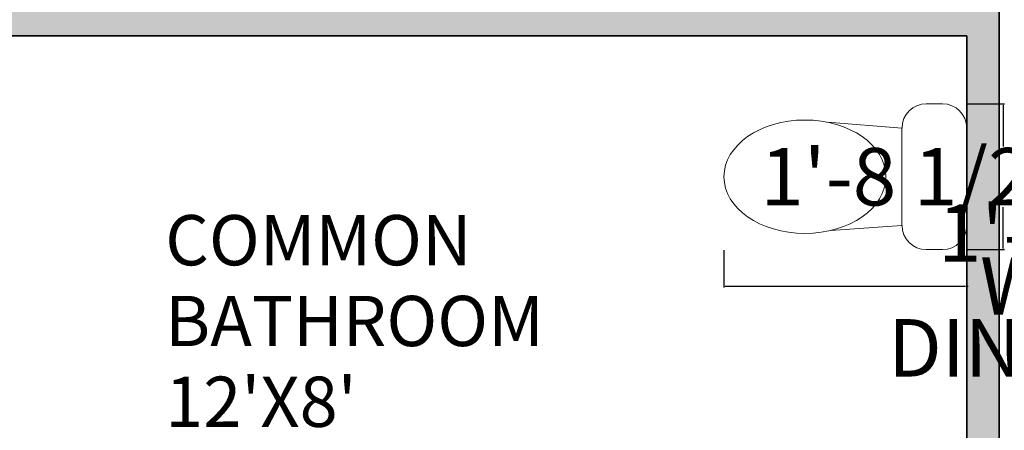
# Model space of a CAD drawing. Units: inches. Extents: x 638 to 1303, y 1 to 699.
# Tile 4 of 21: x 718 to 855, y 252 to 310. Entities that reach past the tile are written whole.
import ezdxf

# ---------------------------------------------------------------- set-up
doc = ezdxf.new("R2010")
doc.units = ezdxf.units.IN
doc.header["$MEASUREMENT"] = 0
for name, color, linetype, lineweight in [('A-ANNO-DIMS', 2, 'Continuous', 18), ('A-AREA-IDEN', 7, 'Continuous', 18), ('A-FLOR-FIXT', 9, 'Continuous', 18), ('A-WALL', 7, 'Continuous', 35)]:
    doc.layers.add(name, color=color, linetype=linetype, lineweight=lineweight)
doc.layers.add('A-WALL-PATT', color=143, linetype='Continuous', lineweight=13, true_color=0x7aafdf)
doc.styles.get("Standard").update_dxf_attribs({"font": 'arial.ttf'})
doc.dimstyles.get("Standard").update_dxf_attribs({"dimtxt": 8, "dimasz": 0.18, "dimexe": 0.18, "dimexo": 0.0625, "dimgap": 0.09, "dimtad": 0, "dimtih": 1, "dimtoh": 1, "dimdec": 4, "dimzin": 0, "dimdsep": 46, "dimlunit": 3, "dimtxsty": 'Standard', "dimcen": 0.09, "dimadec": 0, "dimazin": 0, "dimtfac": 1, "dimtdec": 4, "dimtofl": 0, "dimtmove": 0, "dimatfit": 3, "dimfxl": 1, "dimtolj": 1, "dimtzin": 0, "dimarcsym": 0})

# ---------------------------------------------------------------- blocks, each defined once
blk = doc.blocks.new('WC-CLOSE-COUPLED')
for p, q in [((28.2, 20.3), (30.45, 20.3)), ((24.81, 16.92), (14.41, 17.74)), ((24.81, 3.38), (24.81, 16.92)), ((33.84, 16.92), (33.84, 3.38)), ((24.81, 3.38), (14.9, 2.67)), ((30.45, 0), (28.2, 0))]:
    blk.add_line(p, q)
for centre, start, end in [((28.2, 16.92), 90, 180), ((30.45, 16.92), 0, 90), ((28.2, 3.38), 180, 270), ((30.45, 3.38), 270, 0)]:
    blk.add_arc(centre, 3.38, start, end)
blk.add_ellipse((11.28, 10.15), major_axis=(-11.28, 0), ratio=0.7)
blk = doc.blocks.new('*D30')
at = {"layer": 'A-ANNO-DIMS', "color": 0, "lineweight": -2, "transparency": 16777216}
for p, q in [((913.6, 276.19), (909.79, 276.19)), ((909.97, 276.01), (909.97, 268.11)), ((909.97, 251.76), (909.97, 259.66)), ((913.6, 251.58), (909.79, 251.58))]:
    blk.add_line(p, q, dxfattribs=at)
at = {"layer": 'A-ANNO-DIMS', "color": 0, "transparency": 16777216}
for points in [[(909.94, 276.01), (910, 276.01), (909.97, 276.19)], [(909.94, 251.76), (910, 251.76), (909.97, 251.58)]]:
    blk.add_solid(points, dxfattribs=at)
at = {"layer": 'Defpoints', "color": 0, "transparency": 16777216}
for p in [(913.67, 276.19), (909.97, 251.58), (913.67, 251.58)]:
    blk.add_point(p, dxfattribs=at)
at = {"layer": 'A-ANNO-DIMS', "color": 0, "transparency": 16777216, "insert": (909.97, 263.89), "char_height": 8, "attachment_point": 5}
blk.add_mtext('\\A1;DINING CHAIR 2\'-0 1/2" TYP.', dxfattribs=at)
blk = doc.blocks.new('*D31')
at = {"layer": 'A-ANNO-DIMS', "color": 0, "lineweight": -2, "transparency": 16777216}
for p, q in [((913.67, 279.88), (913.49, 279.88)), ((913.67, 276.25), (913.67, 280.06)), ((934.89, 279.88), (913.85, 279.88)), ((935.07, 276.25), (935.07, 280.06))]:
    blk.add_line(p, q, dxfattribs=at)
at = {"layer": 'A-ANNO-DIMS', "color": 0, "transparency": 16777216}
for points in [[(913.85, 279.91), (913.85, 279.85), (913.67, 279.88)], [(934.89, 279.91), (934.89, 279.85), (935.07, 279.88)]]:
    blk.add_solid(points, dxfattribs=at)
at = {"layer": 'Defpoints', "color": 0, "transparency": 16777216}
for p in [(913.67, 279.88), (913.67, 276.19), (935.07, 276.19)]:
    blk.add_point(p, dxfattribs=at)
at = {"layer": 'A-ANNO-DIMS', "color": 0, "transparency": 16777216, "insert": (880.07, 279.88), "char_height": 8, "attachment_point": 5}
blk.add_mtext('\\A1;1\'-9 1/2" TYP.', dxfattribs=at)
blk = doc.blocks.new('*D32')
at = {"layer": 'A-ANNO-DIMS', "color": 0, "lineweight": -2, "transparency": 16777216}
for p, q in [((816.4, 277.5), (816.4, 272.31)), ((850.23, 277.5), (850.23, 272.31)), ((816.58, 272.49), (850.05, 272.49)), ((850.23, 272.49), (850.41, 272.49))]:
    blk.add_line(p, q, dxfattribs=at)
at = {"layer": 'A-ANNO-DIMS', "color": 0, "transparency": 16777216}
for points in [[(816.58, 272.52), (816.58, 272.46), (816.4, 272.49)], [(850.05, 272.52), (850.05, 272.46), (850.23, 272.49)]]:
    blk.add_solid(points, dxfattribs=at)
at = {"layer": 'Defpoints', "color": 0, "transparency": 16777216}
for p in [(816.4, 277.56), (850.23, 277.56), (850.23, 272.49)]:
    blk.add_point(p, dxfattribs=at)
at = {"layer": 'A-ANNO-DIMS', "color": 0, "transparency": 16777216, "insert": (889.02, 272.49), "char_height": 8, "attachment_point": 5}
blk.add_mtext('\\A1;WC 2\'-10" TYP.', dxfattribs=at)
blk = doc.blocks.new('*D33')
at = {"layer": 'A-ANNO-DIMS', "color": 0, "lineweight": -2, "transparency": 16777216}
for p, q in [((850.3, 297.86), (855.49, 297.86)), ((855.31, 297.68), (855.31, 291.94)), ((855.31, 277.74), (855.31, 283.49)), ((850.3, 277.56), (855.49, 277.56))]:
    blk.add_line(p, q, dxfattribs=at)
at = {"layer": 'A-ANNO-DIMS', "color": 0, "transparency": 16777216}
for points in [[(855.28, 297.68), (855.34, 297.68), (855.31, 297.86)], [(855.28, 277.74), (855.34, 277.74), (855.31, 277.56)]]:
    blk.add_solid(points, dxfattribs=at)
at = {"layer": 'Defpoints', "color": 0, "transparency": 16777216}
for p in [(850.23, 297.86), (855.31, 297.86), (850.23, 277.56)]:
    blk.add_point(p, dxfattribs=at)
at = {"layer": 'A-ANNO-DIMS', "color": 0, "transparency": 16777216, "insert": (855.31, 287.71), "char_height": 8, "attachment_point": 5}
blk.add_mtext('\\A1;1\'-8 1/2" TYP.', dxfattribs=at)

msp = doc.modelspace()

# ---------------------------------------------------------------- hatches: boundary and pattern name
at = {"layer": 'A-WALL-PATT'}
h = msp.add_hatch(color=256, dxfattribs=at)
h.dxf.hatch_style = 1
h.paths.add_polyline_path([(973.34524, 629.81895), (793.35541, 629.81895), (793.35541, 620.81895), (850.23798, 620.81895), (922.23798, 620.81895), (922.23798, 524.81895), (908.94335, 524.81895), (908.94335, 520.31895), (926.73798, 520.31895), (926.73798, 544.31895), (979.3571, 544.31895), (979.3571, 548.81895), (926.73798, 548.81895), (926.73798, 620.81895), (973.34524, 620.81895)])
h.paths.add_polyline_path([(758.35541, 629.81895), (697.23798, 629.81895), (697.23798, 586.77451), (706.23798, 586.77451), (706.23798, 620.81895), (758.35541, 620.81895)])
h.paths.add_polyline_path([(1075.85281, 629.81895), (1003.34524, 629.81895), (1003.34524, 620.81895), (1046.73798, 620.81895), (1046.73798, 560.81895), (1046.73798, 548.81895), (1026.3571, 548.81895), (1026.3571, 544.31895), (1046.73798, 544.31895), (1046.73798, 486.87457), (1051.23798, 486.87457), (1051.23798, 556.31895), (1162.89753, 556.31895), (1162.89753, 560.81895), (1051.23798, 560.81895), (1051.23798, 620.81895), (1075.85281, 620.81895)])
h.paths.add_polyline_path([(1228.23798, 629.81895), (1105.85281, 629.81895), (1105.85281, 620.81895), (1219.23798, 620.81895), (1219.23798, 560.81895), (1197.89753, 560.81895), (1197.89753, 556.31895), (1219.23798, 556.31895), (1219.23798, 498.80084), (1228.23798, 498.80084)])
h.paths.add_polyline_path([(1051.23798, 439.87457), (1046.73798, 439.87457), (1046.73798, 407.81895), (1219.23798, 407.81895), (1219.23798, 381.66175), (1228.23798, 381.66175), (1228.23798, 451.80084), (1219.23798, 451.80084), (1219.23798, 412.31895), (1051.23798, 412.31895)])
h.paths.add_polyline_path([(1228.23798, 346.66175), (1219.23798, 346.66175), (1219.23798, 335.81895), (1046.73798, 335.81895), (1046.73798, 273.56895), (1051.23798, 273.56895), (1051.23798, 331.31895), (1219.23798, 331.31895), (1219.23798, 308.99654), (1228.23798, 308.99654)])
h.paths.add_polyline_path([(1228.23798, 261.99654), (1219.23798, 261.99654), (1219.23798, 211.31895), (1051.23798, 211.31895), (1051.23798, 226.56895), (1046.73798, 226.56895), (1046.73798, 211.31895), (983.84714, 211.31895), (983.84714, 206.81895), (1219.23798, 206.81895), (1219.23798, 166.83987), (1228.23798, 166.83987)])
h.paths.add_polyline_path([(1228.23798, 119.83987), (1219.23798, 119.83987), (1219.23798, 50.81895), (1197.89277, 50.81895), (1197.89277, 41.81895), (1228.23798, 41.81895)])
h.paths.add_polyline_path([(1162.89277, 50.81895), (1069.02949, 50.81895), (1069.02949, 41.81895), (1162.89277, 41.81895)])
h.paths.add_polyline_path([(1010.02949, 50.81895), (941.89631, 50.81895), (917.77455, 50.81895), (917.77455, 41.81895), (941.89631, 41.81895), (1010.02949, 41.81895)])
h.paths.add_polyline_path([(882.77455, 50.81895), (854.73798, 50.81895), (854.73798, 145.50379), (850.23798, 145.50379), (850.23798, 50.81895), (793.49755, 50.81895), (793.49755, 41.81895), (882.77455, 41.81895)])
h.paths.add_polyline_path([(746.49755, 50.81895), (706.23798, 50.81895), (706.23798, 96.57416), (697.23798, 96.57416), (697.23798, 41.81895), (746.49755, 41.81895)])
h.paths.add_polyline_path([(706.23798, 206.81895), (714.01165, 206.81895), (714.01165, 211.31895), (706.23798, 211.31895), (706.23798, 251.21966), (697.23798, 251.21966), (697.23798, 143.57416), (706.23798, 143.57416)])
h.paths.add_polyline_path([(923.84714, 211.31895), (854.73798, 211.31895), (854.73798, 397.8313), (850.23798, 397.8313), (850.23798, 388.31895), (747.9539, 388.31895), (747.9539, 383.81895), (850.23798, 383.81895), (850.23798, 311.81895), (706.23798, 311.81895), (706.23798, 342.78787), (697.23798, 342.78787), (697.23798, 281.21966), (706.23798, 281.21966), (706.23798, 307.31895), (850.23798, 307.31895), (850.23798, 211.31895), (749.01165, 211.31895), (749.01165, 206.81895), (850.23798, 206.81895), (850.23798, 192.50379), (854.73798, 192.50379), (854.73798, 206.81895), (923.84714, 206.81895)])
h.paths.add_polyline_path([(706.23798, 434.70471), (697.23798, 434.70471), (697.23798, 372.78787), (706.23798, 372.78787), (706.23798, 383.81895), (712.9539, 383.81895), (712.9539, 388.31895), (706.23798, 388.31895)])
h.paths.add_polyline_path([(706.23798, 520.31895), (850.23798, 520.31895), (850.23798, 444.8313), (854.73798, 444.8313), (854.73798, 520.31895), (861.94335, 520.31895), (861.94335, 524.81895), (706.23798, 524.81895), (706.23798, 551.77451), (697.23798, 551.77451), (697.23798, 481.70471), (706.23798, 481.70471)])

# ---------------------------------------------------------------- linework, layer by layer
at = {"layer": 'A-WALL'}
for p, q in [((854.73798, 211.31895), (854.73798, 397.8313)), ((850.23798, 307.31895), (706.23798, 307.31895)), ((850.23798, 211.31895), (850.23798, 307.31895))]:
    msp.add_line(p, q, dxfattribs=at)

# ---------------------------------------------------------------- block references
at = {"layer": 'A-FLOR-FIXT'}
msp.add_blockref('WC-CLOSE-COUPLED', (816.399, 277.561), dxfattribs=at)

# ---------------------------------------------------------------- texts
at = {"layer": 'A-AREA-IDEN'}
for s, p in [('COMMON ', (738.55699, 275.37654)), ('BATHROOM', (738.55699, 264.13166)), ("12'X8'", (738.55699, 252.88678))]:
    msp.add_text(s, height=7, dxfattribs=at).set_placement(p)

# ---------------------------------------------------------------- dimensions: what is measured, and where the dimension line sits
at = {"layer": 'A-ANNO-DIMS'}
for base, p1, p2, angle, text, picture, middle in [((855.31003, 297.86284), (850.23465, 277.56133), (850.23465, 297.86284), 90, '<> TYP.', '*D33', (855.31003, 287.71209)), ((913.66615, 279.88354), (935.07007, 276.19196), (913.66615, 276.19196), 180, '<> TYP.', '*D31', (880.0701, 279.88354)), ((909.97457, 251.58144), (913.66615, 276.19196), (913.66615, 251.58144), 270, 'DINING CHAIR <> TYP.', '*D30', (909.97457, 263.8867))]:
    dim = msp.add_linear_dim(base=base, p1=p1, p2=p2, angle=angle, text=text, dimstyle='Standard', override={"dimdec": 1, "dimlfac": 1, "dimrnd": 0, "dimzin": 1, "dimdsep": 46, "dimlunit": 4, "dimfrac": 2}, dxfattribs=at)
    dim.commit()
    dim.dimension.update_dxf_attribs({"geometry": picture, "text_midpoint": middle})
dim = msp.add_linear_dim(base=(850.23465, 272.48596), p1=(816.39881, 277.56133), p2=(850.23465, 277.56133), text='WC <> TYP.', dimstyle='Standard', override={"dimdec": 1, "dimlfac": 1, "dimrnd": 0, "dimzin": 1, "dimdsep": 46, "dimlunit": 4, "dimfrac": 2}, dxfattribs=at)
dim.commit()
dim.dimension.update_dxf_attribs({"geometry": '*D32', "text_midpoint": (889.02034, 272.48596)})

doc.saveas('drawing.dxf')
